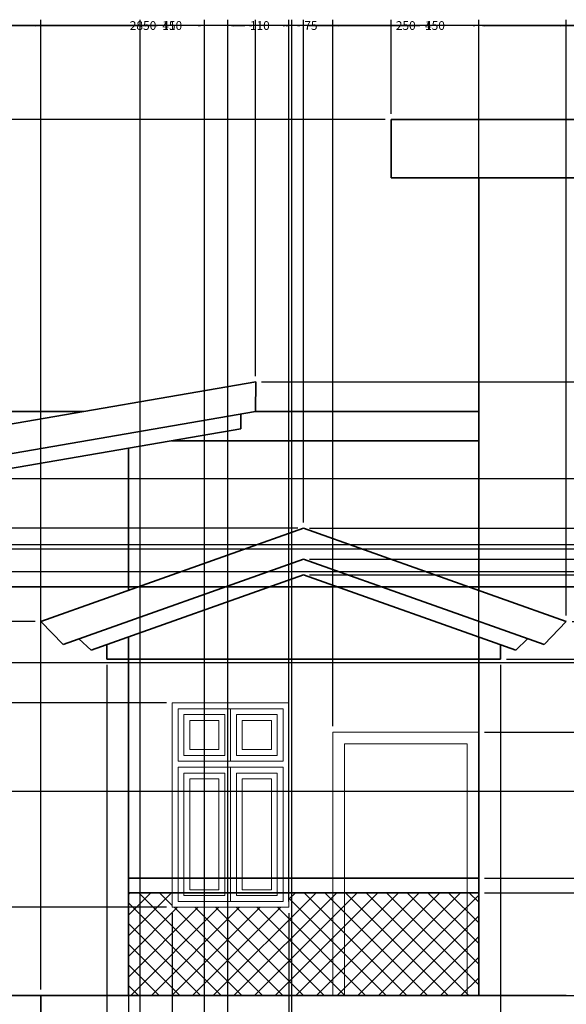
# Model space of a CAD drawing. Units: millimetres. Extents: x 937 to 4561, y 2711 to 5748.
# Tile 7 of 8: x 2543 to 3479, y 4062 to 5748. Entities that reach past the tile are written whole.
import ezdxf

# ---------------------------------------------------------------- set-up
doc = ezdxf.new("R2010")
doc.units = ezdxf.units.MM
doc.header["$MEASUREMENT"] = 0
for name, color, linetype, lineweight in [('A-ANNO-DIMS', 2, 'Continuous', 18), ('A-DOOR', 3, 'Continuous', 18), ('A-ELEV', 7, 'Continuous', 35), ('A-GLAZ', 4, 'Continuous', 18), ('A-ROOF', 1, 'Continuous', 35), ('A-WALL-PATT', 8, 'Continuous', 13)]:
    doc.layers.add(name, color=color, linetype=linetype, lineweight=lineweight)
doc.styles.get("Standard").update_dxf_attribs({"font": 'arial.ttf'})
doc.dimstyles.get("Standard").update_dxf_attribs({"dimtxt": 15, "dimasz": 10, "dimexe": 10, "dimexo": 10, "dimgap": 10, "dimtad": 0, "dimtih": 1, "dimtoh": 1, "dimdec": 0, "dimzin": 0, "dimdsep": 46, "dimtxsty": 'Standard', "dimcen": 5, "dimadec": 0, "dimazin": 0, "dimtfac": 1, "dimtdec": 0, "dimtofl": 0, "dimtmove": 0, "dimatfit": 3, "dimfxl": 1, "dimtolj": 1, "dimtzin": 0, "dimarcsym": 0})

# ---------------------------------------------------------------- blocks, each defined once
blk = doc.blocks.new('*D15')
at = {"layer": 'A-ANNO-DIMS', "color": 0, "lineweight": -2, "transparency": 16777216}
for p, q in [((1329.5, 4086.9), (1329.5, 5747.9)), ((1339.5, 5737.9), (2722, 5737.9)), ((4169.5, 5737.9), (2787, 5737.9)), ((4179.5, 5586.9), (4179.5, 5747.9))]:
    blk.add_line(p, q, dxfattribs=at)
at = {"layer": 'A-ANNO-DIMS', "color": 0, "transparency": 16777216}
for points in [[(1339.5, 5739.6), (1339.5, 5736.2), (1329.5, 5737.9)], [(4169.5, 5739.6), (4169.5, 5736.2), (4179.5, 5737.9)]]:
    blk.add_solid(points, dxfattribs=at)
at = {"layer": 'Defpoints', "color": 0, "transparency": 16777216}
for p in [(4179.5, 5737.9), (4179.5, 5576.9), (1329.5, 4076.9)]:
    blk.add_point(p, dxfattribs=at)
at = {"layer": 'A-ANNO-DIMS', "color": 0, "transparency": 16777216, "insert": (2754.5, 5737.9), "char_height": 15, "attachment_point": 5}
blk.add_mtext('\\A1;2850', dxfattribs=at)
blk = doc.blocks.new('*D16')
at = {"layer": 'A-ANNO-DIMS', "color": 0, "lineweight": -2, "transparency": 16777216}
for p, q in [((1329.5, 4859.2), (1329.5, 5747.9)), ((1339.5, 5737.9), (2106.8, 5737.9)), ((2937.4, 5737.9), (2170.2, 5737.9)), ((2947.4, 5137.7), (2947.4, 5747.9))]:
    blk.add_line(p, q, dxfattribs=at)
at = {"layer": 'A-ANNO-DIMS', "color": 0, "transparency": 16777216}
for points in [[(1339.5, 5739.6), (1339.5, 5736.2), (1329.5, 5737.9)], [(2937.4, 5739.6), (2937.4, 5736.2), (2947.4, 5737.9)]]:
    blk.add_solid(points, dxfattribs=at)
at = {"layer": 'Defpoints', "color": 0, "transparency": 16777216}
for p in [(2947.4, 5737.9), (2947.4, 5127.7), (1329.5, 4849.2)]:
    blk.add_point(p, dxfattribs=at)
at = {"layer": 'A-ANNO-DIMS', "color": 0, "transparency": 16777216, "insert": (2138.5, 5737.9), "char_height": 15, "attachment_point": 5}
blk.add_mtext('\\A1;1618', dxfattribs=at)
blk = doc.blocks.new('*D17')
at = {"layer": 'A-ANNO-DIMS', "color": 0, "lineweight": -2, "transparency": 16777216}
for p, q in [((3179.5, 5586.9), (3179.5, 5747.9)), ((3189.5, 5737.9), (3228.6, 5737.9)), ((3319.5, 5737.9), (3280.3, 5737.9)), ((3329.5, 5486.9), (3329.5, 5747.9))]:
    blk.add_line(p, q, dxfattribs=at)
at = {"layer": 'A-ANNO-DIMS', "color": 0, "transparency": 16777216}
for points in [[(3189.5, 5739.6), (3189.5, 5736.2), (3179.5, 5737.9)], [(3319.5, 5739.6), (3319.5, 5736.2), (3329.5, 5737.9)]]:
    blk.add_solid(points, dxfattribs=at)
at = {"layer": 'Defpoints', "color": 0, "transparency": 16777216}
for p in [(3329.5, 5737.9), (3179.5, 5576.9), (3329.5, 5476.9)]:
    blk.add_point(p, dxfattribs=at)
at = {"layer": 'A-ANNO-DIMS', "color": 0, "transparency": 16777216, "insert": (3254.5, 5737.9), "char_height": 15, "attachment_point": 5}
blk.add_mtext('\\A1;150', dxfattribs=at)
blk = doc.blocks.new('*D18')
at = {"layer": 'A-ANNO-DIMS', "color": 0, "lineweight": -2, "transparency": 16777216}
for p, q in [((3329.5, 5486.9), (3329.5, 5747.9)), ((3339.5, 5737.9), (3653, 5737.9)), ((4019.5, 5737.9), (3706, 5737.9)), ((4029.5, 5486.9), (4029.5, 5747.9))]:
    blk.add_line(p, q, dxfattribs=at)
at = {"layer": 'A-ANNO-DIMS', "color": 0, "transparency": 16777216}
for points in [[(3339.5, 5739.6), (3339.5, 5736.2), (3329.5, 5737.9)], [(4019.5, 5739.6), (4019.5, 5736.2), (4029.5, 5737.9)]]:
    blk.add_solid(points, dxfattribs=at)
at = {"layer": 'Defpoints', "color": 0, "transparency": 16777216}
for p in [(4029.5, 5737.9), (3329.5, 5476.9), (4029.5, 5476.9)]:
    blk.add_point(p, dxfattribs=at)
at = {"layer": 'A-ANNO-DIMS', "color": 0, "transparency": 16777216, "insert": (3679.5, 5737.9), "char_height": 15, "attachment_point": 5}
blk.add_mtext('\\A1;700', dxfattribs=at)
blk = doc.blocks.new('*D22')
at = {"layer": 'A-ANNO-DIMS', "color": 0, "lineweight": -2, "transparency": 16777216}
for p, q in [((2579.5, 4727.5), (2579.5, 5747.9)), ((2589.5, 5737.9), (2777.6, 5737.9)), ((3019.5, 5737.9), (2831.3, 5737.9)), ((3029.5, 4886.9), (3029.5, 5747.9))]:
    blk.add_line(p, q, dxfattribs=at)
at = {"layer": 'A-ANNO-DIMS', "color": 0, "transparency": 16777216}
for points in [[(2589.5, 5739.6), (2589.5, 5736.2), (2579.5, 5737.9)], [(3019.5, 5739.6), (3019.5, 5736.2), (3029.5, 5737.9)]]:
    blk.add_solid(points, dxfattribs=at)
at = {"layer": 'Defpoints', "color": 0, "transparency": 16777216}
for p in [(3029.5, 5737.9), (3029.5, 4876.9), (2579.5, 4717.5)]:
    blk.add_point(p, dxfattribs=at)
at = {"layer": 'A-ANNO-DIMS', "color": 0, "transparency": 16777216, "insert": (2804.5, 5737.9), "char_height": 15, "attachment_point": 5}
blk.add_mtext('\\A1;450', dxfattribs=at)
blk = doc.blocks.new('*D23')
at = {"layer": 'A-ANNO-DIMS', "color": 0, "lineweight": -2, "transparency": 16777216}
for p, q in [((3029.5, 4886.9), (3029.5, 5747.9)), ((3039.5, 5737.9), (3227.6, 5737.9)), ((3469.5, 5737.9), (3281.3, 5737.9)), ((3479.5, 4727.5), (3479.5, 5747.9))]:
    blk.add_line(p, q, dxfattribs=at)
at = {"layer": 'A-ANNO-DIMS', "color": 0, "transparency": 16777216}
for points in [[(3039.5, 5739.6), (3039.5, 5736.2), (3029.5, 5737.9)], [(3469.5, 5739.6), (3469.5, 5736.2), (3479.5, 5737.9)]]:
    blk.add_solid(points, dxfattribs=at)
at = {"layer": 'Defpoints', "color": 0, "transparency": 16777216}
for p in [(3479.5, 5737.9), (3029.5, 4876.9), (3479.5, 4717.5)]:
    blk.add_point(p, dxfattribs=at)
at = {"layer": 'A-ANNO-DIMS', "color": 0, "transparency": 16777216, "insert": (3254.5, 5737.9), "char_height": 15, "attachment_point": 5}
blk.add_mtext('\\A1;450', dxfattribs=at)
blk = doc.blocks.new('*D24')
at = {"layer": 'A-ANNO-DIMS', "color": 0, "lineweight": -2, "transparency": 16777216}
for p, q in [((2692.4, 4642.9), (2692.4, 2710.9)), ((3366.9, 4642.9), (3366.9, 2710.9)), ((2702.4, 2720.9), (2994.3, 2720.9)), ((3356.9, 2720.9), (3065.1, 2720.9))]:
    blk.add_line(p, q, dxfattribs=at)
at = {"layer": 'A-ANNO-DIMS', "color": 0, "transparency": 16777216}
for points in [[(2702.4, 2722.6), (2702.4, 2719.2), (2692.4, 2720.9)], [(3356.9, 2722.6), (3356.9, 2719.2), (3366.9, 2720.9)]]:
    blk.add_solid(points, dxfattribs=at)
at = {"layer": 'Defpoints', "color": 0, "transparency": 16777216}
for p in [(2692.4, 4652.9), (3366.9, 4652.9), (3366.9, 2720.9)]:
    blk.add_point(p, dxfattribs=at)
at = {"layer": 'A-ANNO-DIMS', "color": 0, "transparency": 16777216, "insert": (3029.7, 2720.9), "char_height": 15, "attachment_point": 5}
blk.add_mtext('\\A1;674.5', dxfattribs=at)
blk = doc.blocks.new('*D25')
at = {"layer": 'A-ANNO-DIMS', "color": 0, "lineweight": -2, "transparency": 16777216}
for p, q in [((3469.5, 5737.9), (3459.5, 5737.9)), ((3479.5, 5086.9), (3479.5, 5747.9)), ((3529.5, 5036.9), (3529.5, 5747.9)), ((3539.5, 5737.9), (3549.5, 5737.9))]:
    blk.add_line(p, q, dxfattribs=at)
at = {"layer": 'A-ANNO-DIMS', "color": 0, "transparency": 16777216}
for points in [[(3469.5, 5739.6), (3469.5, 5736.2), (3479.5, 5737.9)], [(3539.5, 5739.6), (3539.5, 5736.2), (3529.5, 5737.9)]]:
    blk.add_solid(points, dxfattribs=at)
at = {"layer": 'Defpoints', "color": 0, "transparency": 16777216}
for p in [(3529.5, 5737.9), (3479.5, 5076.9), (3529.5, 5026.9)]:
    blk.add_point(p, dxfattribs=at)
at = {"layer": 'A-ANNO-DIMS', "color": 0, "transparency": 16777216, "insert": (3504.5, 5737.9), "char_height": 15, "attachment_point": 5}
blk.add_mtext('\\A1;50', dxfattribs=at)
blk = doc.blocks.new('*D43')
at = {"layer": 'A-ANNO-DIMS', "color": 0, "lineweight": -2, "transparency": 16777216}
for p, q in [((1329.5, 4086.9), (1329.5, 5747.9)), ((1339.5, 5737.9), (1922.8, 5737.9)), ((2569.5, 5737.9), (1986.2, 5737.9)), ((2579.5, 4086.9), (2579.5, 5747.9))]:
    blk.add_line(p, q, dxfattribs=at)
at = {"layer": 'A-ANNO-DIMS', "color": 0, "transparency": 16777216}
for points in [[(1339.5, 5739.6), (1339.5, 5736.2), (1329.5, 5737.9)], [(2569.5, 5739.6), (2569.5, 5736.2), (2579.5, 5737.9)]]:
    blk.add_solid(points, dxfattribs=at)
at = {"layer": 'Defpoints', "color": 0, "transparency": 16777216}
for p in [(2579.5, 5737.9), (1329.5, 4076.9), (2579.5, 4076.9)]:
    blk.add_point(p, dxfattribs=at)
at = {"layer": 'A-ANNO-DIMS', "color": 0, "transparency": 16777216, "insert": (1954.5, 5737.9), "char_height": 15, "attachment_point": 5}
blk.add_mtext('\\A1;1250', dxfattribs=at)
blk = doc.blocks.new('*D49')
at = {"layer": 'A-ANNO-DIMS', "color": 0, "lineweight": -2, "transparency": 16777216}
for p, q in [((2729.5, 4242.9), (2729.5, 2710.9)), ((2804.5, 4217.9), (2804.5, 2710.9)), ((2719.5, 2720.9), (2709.5, 2720.9)), ((2814.5, 2720.9), (2824.5, 2720.9))]:
    blk.add_line(p, q, dxfattribs=at)
at = {"layer": 'A-ANNO-DIMS', "color": 0, "transparency": 16777216}
for points in [[(2719.5, 2722.6), (2719.5, 2719.2), (2729.5, 2720.9)], [(2814.5, 2722.6), (2814.5, 2719.2), (2804.5, 2720.9)]]:
    blk.add_solid(points, dxfattribs=at)
at = {"layer": 'Defpoints', "color": 0, "transparency": 16777216}
for p in [(2729.5, 4252.9), (2804.5, 4227.9), (2804.5, 2720.9)]:
    blk.add_point(p, dxfattribs=at)
at = {"layer": 'A-ANNO-DIMS', "color": 0, "transparency": 16777216, "insert": (2767, 2720.9), "char_height": 15, "attachment_point": 5}
blk.add_mtext('\\A1;75', dxfattribs=at)
blk = doc.blocks.new('*D50')
at = {"layer": 'A-ANNO-DIMS', "color": 0, "lineweight": -2, "transparency": 16777216}
for p, q in [((2804.5, 4217.9), (2804.5, 2710.9)), ((3004.5, 4217.9), (3004.5, 2710.9)), ((2814.5, 2720.9), (2877.8, 2720.9)), ((2994.5, 2720.9), (2931.2, 2720.9))]:
    blk.add_line(p, q, dxfattribs=at)
at = {"layer": 'A-ANNO-DIMS', "color": 0, "transparency": 16777216}
for points in [[(2814.5, 2722.6), (2814.5, 2719.2), (2804.5, 2720.9)], [(2994.5, 2722.6), (2994.5, 2719.2), (3004.5, 2720.9)]]:
    blk.add_solid(points, dxfattribs=at)
at = {"layer": 'Defpoints', "color": 0, "transparency": 16777216}
for p in [(2804.5, 4227.9), (3004.5, 4227.9), (3004.5, 2720.9)]:
    blk.add_point(p, dxfattribs=at)
at = {"layer": 'A-ANNO-DIMS', "color": 0, "transparency": 16777216, "insert": (2904.5, 2720.9), "char_height": 15, "attachment_point": 5}
blk.add_mtext('\\A1;200', dxfattribs=at)
blk = doc.blocks.new('*D51')
at = {"layer": 'A-ANNO-DIMS', "color": 0, "lineweight": -2, "transparency": 16777216}
for p, q in [((2994.5, 5737.9), (2984.5, 5737.9)), ((3004.5, 4237.9), (3004.5, 5747.9)), ((3079.5, 4537.9), (3079.5, 5747.9)), ((3089.5, 5737.9), (3099.5, 5737.9))]:
    blk.add_line(p, q, dxfattribs=at)
at = {"layer": 'A-ANNO-DIMS', "color": 0, "transparency": 16777216}
for points in [[(2994.5, 5739.6), (2994.5, 5736.2), (3004.5, 5737.9)], [(3089.5, 5739.6), (3089.5, 5736.2), (3079.5, 5737.9)]]:
    blk.add_solid(points, dxfattribs=at)
at = {"layer": 'Defpoints', "color": 0, "transparency": 16777216}
for p in [(3079.5, 5737.9), (3079.5, 4527.9), (3004.5, 4227.9)]:
    blk.add_point(p, dxfattribs=at)
at = {"layer": 'A-ANNO-DIMS', "color": 0, "transparency": 16777216, "insert": (3042, 5737.9), "char_height": 15, "attachment_point": 5}
blk.add_mtext('\\A1;75', dxfattribs=at)
blk = doc.blocks.new('*D52')
at = {"layer": 'A-ANNO-DIMS', "color": 0, "lineweight": -2, "transparency": 16777216}
for p, q in [((3079.5, 4537.9), (3079.5, 5747.9)), ((3089.5, 5737.9), (3177.8, 5737.9)), ((3319.5, 5737.9), (3231.2, 5737.9)), ((3329.5, 4537.9), (3329.5, 5747.9))]:
    blk.add_line(p, q, dxfattribs=at)
at = {"layer": 'A-ANNO-DIMS', "color": 0, "transparency": 16777216}
for points in [[(3089.5, 5739.6), (3089.5, 5736.2), (3079.5, 5737.9)], [(3319.5, 5739.6), (3319.5, 5736.2), (3329.5, 5737.9)]]:
    blk.add_solid(points, dxfattribs=at)
at = {"layer": 'Defpoints', "color": 0, "transparency": 16777216}
for p in [(3329.5, 5737.9), (3079.5, 4527.9), (3329.5, 4527.9)]:
    blk.add_point(p, dxfattribs=at)
at = {"layer": 'A-ANNO-DIMS', "color": 0, "transparency": 16777216, "insert": (3204.5, 5737.9), "char_height": 15, "attachment_point": 5}
blk.add_mtext('\\A1;250', dxfattribs=at)
blk = doc.blocks.new('*D53')
at = {"layer": 'A-ANNO-DIMS', "color": 0, "lineweight": -2, "transparency": 16777216}
for p, q in [((2749.5, 3666.9), (2749.5, 5747.9)), ((2759.5, 5737.9), (2778.6, 5737.9)), ((2849.5, 5737.9), (2830.3, 5737.9)), ((2859.5, 3666.9), (2859.5, 5747.9))]:
    blk.add_line(p, q, dxfattribs=at)
at = {"layer": 'A-ANNO-DIMS', "color": 0, "transparency": 16777216}
for points in [[(2759.5, 5739.6), (2759.5, 5736.2), (2749.5, 5737.9)], [(2849.5, 5739.6), (2849.5, 5736.2), (2859.5, 5737.9)]]:
    blk.add_solid(points, dxfattribs=at)
at = {"layer": 'Defpoints', "color": 0, "transparency": 16777216}
for p in [(2859.5, 5737.9), (2749.5, 3656.9), (2859.5, 3656.9)]:
    blk.add_point(p, dxfattribs=at)
at = {"layer": 'A-ANNO-DIMS', "color": 0, "transparency": 16777216, "insert": (2804.5, 5737.9), "char_height": 15, "attachment_point": 5}
blk.add_mtext('\\A1;110', dxfattribs=at)
blk = doc.blocks.new('*D54')
at = {"layer": 'A-ANNO-DIMS', "color": 0, "lineweight": -2, "transparency": 16777216}
for p, q in [((2899.5, 3666.9), (2899.5, 5747.9)), ((2909.5, 5737.9), (2928.6, 5737.9)), ((2999.5, 5737.9), (2980.3, 5737.9)), ((3009.5, 3666.9), (3009.5, 5747.9))]:
    blk.add_line(p, q, dxfattribs=at)
at = {"layer": 'A-ANNO-DIMS', "color": 0, "transparency": 16777216}
for points in [[(2909.5, 5739.6), (2909.5, 5736.2), (2899.5, 5737.9)], [(2999.5, 5739.6), (2999.5, 5736.2), (3009.5, 5737.9)]]:
    blk.add_solid(points, dxfattribs=at)
at = {"layer": 'Defpoints', "color": 0, "transparency": 16777216}
for p in [(3009.5, 5737.9), (2899.5, 3656.9), (3009.5, 3656.9)]:
    blk.add_point(p, dxfattribs=at)
at = {"layer": 'A-ANNO-DIMS', "color": 0, "transparency": 16777216, "insert": (2954.5, 5737.9), "char_height": 15, "attachment_point": 5}
blk.add_mtext('\\A1;110', dxfattribs=at)
blk = doc.blocks.new('*D63')
at = {"layer": 'A-ANNO-DIMS', "color": 0, "lineweight": -2, "transparency": 16777216}
for p, q in [((3169.5, 5576.9), (958.5, 5576.9)), ((968.5, 5566.9), (968.5, 5344.6)), ((968.5, 5086.9), (968.5, 5309.2)), ((1419.5, 5076.9), (958.5, 5076.9))]:
    blk.add_line(p, q, dxfattribs=at)
at = {"layer": 'A-ANNO-DIMS', "color": 0, "transparency": 16777216}
for points in [[(966.8, 5566.9), (970.2, 5566.9), (968.5, 5576.9)], [(966.8, 5086.9), (970.2, 5086.9), (968.5, 5076.9)]]:
    blk.add_solid(points, dxfattribs=at)
at = {"layer": 'Defpoints', "color": 0, "transparency": 16777216}
for p in [(968.5, 5576.9), (3179.5, 5576.9), (1429.5, 5076.9)]:
    blk.add_point(p, dxfattribs=at)
at = {"layer": 'A-ANNO-DIMS', "color": 0, "transparency": 16777216, "insert": (968.5, 5326.9), "char_height": 15, "attachment_point": 5}
blk.add_mtext('\\A1;500', dxfattribs=at)
blk = doc.blocks.new('*D68')
at = {"layer": 'A-ANNO-DIMS', "color": 0, "lineweight": -2, "transparency": 16777216}
for p, q in [((4490.5, 4812.8), (4490.5, 4822.8)), ((4490.5, 4822.8), (4500.5, 4822.8)), ((1364.5, 4802.8), (4500.5, 4802.8)), ((1364.5, 4777.4), (4500.5, 4777.4)), ((4490.5, 4767.4), (4490.5, 4757.4))]:
    blk.add_line(p, q, dxfattribs=at)
at = {"layer": 'A-ANNO-DIMS', "color": 0, "transparency": 16777216}
for points in [[(4488.8, 4812.8), (4492.2, 4812.8), (4490.5, 4802.8)], [(4488.8, 4767.4), (4492.2, 4767.4), (4490.5, 4777.4)]]:
    blk.add_solid(points, dxfattribs=at)
at = {"layer": 'Defpoints', "color": 0, "transparency": 16777216}
for p in [(1354.5, 4802.8), (4490.5, 4802.8), (1354.5, 4777.4)]:
    blk.add_point(p, dxfattribs=at)
at = {"layer": 'A-ANNO-DIMS', "color": 0, "transparency": 16777216, "insert": (4535.9, 4822.8), "char_height": 15, "attachment_point": 5}
blk.add_mtext('\\A1;25.37', dxfattribs=at)
blk = doc.blocks.new('*D69')
at = {"layer": 'A-ANNO-DIMS', "color": 0, "lineweight": -2, "transparency": 16777216}
for p, q in [((2957.4, 5127.7), (4500.5, 5127.7)), ((4490.5, 5117.7), (4490.5, 5006.1)), ((4490.5, 4859.2), (4490.5, 4970.8)), ((1339.5, 4849.2), (4500.5, 4849.2))]:
    blk.add_line(p, q, dxfattribs=at)
at = {"layer": 'A-ANNO-DIMS', "color": 0, "transparency": 16777216}
for points in [[(4488.8, 5117.7), (4492.2, 5117.7), (4490.5, 5127.7)], [(4488.8, 4859.2), (4492.2, 4859.2), (4490.5, 4849.2)]]:
    blk.add_solid(points, dxfattribs=at)
at = {"layer": 'Defpoints', "color": 0, "transparency": 16777216}
for p in [(2947.4, 5127.7), (4490.5, 5127.7), (1329.5, 4849.2)]:
    blk.add_point(p, dxfattribs=at)
at = {"layer": 'A-ANNO-DIMS', "color": 0, "transparency": 16777216, "insert": (4490.5, 4988.5), "char_height": 15, "attachment_point": 5}
blk.add_mtext('\\A1;278.45', dxfattribs=at)
blk = doc.blocks.new('*D75')
at = {"layer": 'A-ANNO-DIMS', "color": 0, "lineweight": -2, "transparency": 16777216}
for p, q in [((1829.5, 4646.9), (4500.5, 4646.9)), ((4490.5, 4636.9), (4490.5, 4554.6)), ((4490.5, 4436.9), (4490.5, 4519.2)), ((1829.5, 4426.9), (4500.5, 4426.9))]:
    blk.add_line(p, q, dxfattribs=at)
at = {"layer": 'A-ANNO-DIMS', "color": 0, "transparency": 16777216}
for points in [[(4488.8, 4636.9), (4492.2, 4636.9), (4490.5, 4646.9)], [(4488.8, 4436.9), (4492.2, 4436.9), (4490.5, 4426.9)]]:
    blk.add_solid(points, dxfattribs=at)
at = {"layer": 'Defpoints', "color": 0, "transparency": 16777216}
for p in [(1819.5, 4646.9), (4490.5, 4646.9), (1819.5, 4426.9)]:
    blk.add_point(p, dxfattribs=at)
at = {"layer": 'A-ANNO-DIMS', "color": 0, "transparency": 16777216, "insert": (4490.5, 4536.9), "char_height": 15, "attachment_point": 5}
blk.add_mtext('\\A1;220', dxfattribs=at)
blk = doc.blocks.new('*D76')
at = {"layer": 'A-ANNO-DIMS', "color": 0, "lineweight": -2, "transparency": 16777216}
for p, q in [((1829.5, 4776.9), (4500.5, 4776.9)), ((4490.5, 4766.9), (4490.5, 4729.6)), ((4490.5, 4656.9), (4490.5, 4694.2)), ((1829.5, 4646.9), (4500.5, 4646.9))]:
    blk.add_line(p, q, dxfattribs=at)
at = {"layer": 'A-ANNO-DIMS', "color": 0, "transparency": 16777216}
for points in [[(4488.8, 4766.9), (4492.2, 4766.9), (4490.5, 4776.9)], [(4488.8, 4656.9), (4492.2, 4656.9), (4490.5, 4646.9)]]:
    blk.add_solid(points, dxfattribs=at)
at = {"layer": 'Defpoints', "color": 0, "transparency": 16777216}
for p in [(1819.5, 4776.9), (4490.5, 4776.9), (1819.5, 4646.9)]:
    blk.add_point(p, dxfattribs=at)
at = {"layer": 'A-ANNO-DIMS', "color": 0, "transparency": 16777216, "insert": (4490.5, 4711.9), "char_height": 15, "attachment_point": 5}
blk.add_mtext('\\A1;130', dxfattribs=at)
blk = doc.blocks.new('*D78')
at = {"layer": 'A-ANNO-DIMS', "color": 0, "lineweight": -2, "transparency": 16777216}
for p, q in [((2439.5, 4962.4), (4500.5, 4962.4)), ((4490.5, 4952.4), (4490.5, 4919.9)), ((4490.5, 4852), (4490.5, 4884.5)), ((1739.5, 4842), (4500.5, 4842))]:
    blk.add_line(p, q, dxfattribs=at)
at = {"layer": 'A-ANNO-DIMS', "color": 0, "transparency": 16777216}
for points in [[(4488.8, 4952.4), (4492.2, 4952.4), (4490.5, 4962.4)], [(4488.8, 4852), (4492.2, 4852), (4490.5, 4842)]]:
    blk.add_solid(points, dxfattribs=at)
at = {"layer": 'Defpoints', "color": 0, "transparency": 16777216}
for p in [(2429.5, 4962.4), (4490.5, 4962.4), (1729.5, 4842)]:
    blk.add_point(p, dxfattribs=at)
at = {"layer": 'A-ANNO-DIMS', "color": 0, "transparency": 16777216, "insert": (4490.5, 4902.2), "char_height": 15, "attachment_point": 5}
blk.add_mtext('\\A1;120.47', dxfattribs=at)
blk = doc.blocks.new('*D79')
at = {"layer": 'A-ANNO-DIMS', "color": 0, "lineweight": -2, "transparency": 16777216}
for p, q in [((3019.5, 4876.9), (958.5, 4876.9)), ((968.5, 4866.9), (968.5, 4814.8)), ((968.5, 4727.5), (968.5, 4779.5)), ((2569.5, 4717.5), (958.5, 4717.5))]:
    blk.add_line(p, q, dxfattribs=at)
at = {"layer": 'A-ANNO-DIMS', "color": 0, "transparency": 16777216}
for points in [[(966.8, 4866.9), (970.2, 4866.9), (968.5, 4876.9)], [(966.8, 4727.5), (970.2, 4727.5), (968.5, 4717.5)]]:
    blk.add_solid(points, dxfattribs=at)
at = {"layer": 'Defpoints', "color": 0, "transparency": 16777216}
for p in [(968.5, 4876.9), (3029.5, 4876.9), (2579.5, 4717.5)]:
    blk.add_point(p, dxfattribs=at)
at = {"layer": 'A-ANNO-DIMS', "color": 0, "transparency": 16777216, "insert": (968.5, 4797.2), "char_height": 15, "attachment_point": 5}
blk.add_mtext('\\A1;159.44', dxfattribs=at)
blk = doc.blocks.new('*D80')
at = {"layer": 'A-ANNO-DIMS', "color": 0, "lineweight": -2, "transparency": 16777216}
for p, q in [((3039.5, 4876.9), (4500.5, 4876.9)), ((4490.5, 4866.9), (4490.5, 4833.9)), ((3039.5, 4823.9), (4500.5, 4823.9)), ((4490.5, 4823.9), (4490.5, 4813.9)), ((4490.5, 4813.9), (4480.5, 4813.9))]:
    blk.add_line(p, q, dxfattribs=at)
at = {"layer": 'A-ANNO-DIMS', "color": 0, "transparency": 16777216}
for points in [[(4488.8, 4866.9), (4492.2, 4866.9), (4490.5, 4876.9)], [(4488.8, 4833.9), (4492.2, 4833.9), (4490.5, 4823.9)]]:
    blk.add_solid(points, dxfattribs=at)
at = {"layer": 'Defpoints', "color": 0, "transparency": 16777216}
for p in [(3029.5, 4876.9), (3029.5, 4823.9), (4490.5, 4823.9)]:
    blk.add_point(p, dxfattribs=at)
at = {"layer": 'A-ANNO-DIMS', "color": 0, "transparency": 16777216, "insert": (4445.1, 4813.9), "char_height": 15, "attachment_point": 5}
blk.add_mtext('\\A1;53.05', dxfattribs=at)
blk = doc.blocks.new('*D81')
at = {"layer": 'A-ANNO-DIMS', "color": 0, "lineweight": -2, "transparency": 16777216}
for p, q in [((4490.5, 4833.9), (4490.5, 4843.9)), ((3039.5, 4823.9), (4500.5, 4823.9)), ((3039.5, 4797.3), (4500.5, 4797.3)), ((4490.5, 4777.3), (4480.5, 4777.3)), ((4490.5, 4787.3), (4490.5, 4777.3))]:
    blk.add_line(p, q, dxfattribs=at)
at = {"layer": 'A-ANNO-DIMS', "color": 0, "transparency": 16777216}
for points in [[(4488.8, 4833.9), (4492.2, 4833.9), (4490.5, 4823.9)], [(4488.8, 4787.3), (4492.2, 4787.3), (4490.5, 4797.3)]]:
    blk.add_solid(points, dxfattribs=at)
at = {"layer": 'Defpoints', "color": 0, "transparency": 16777216}
for p in [(3029.5, 4823.9), (3029.5, 4797.3), (4490.5, 4797.3)]:
    blk.add_point(p, dxfattribs=at)
at = {"layer": 'A-ANNO-DIMS', "color": 0, "transparency": 16777216, "insert": (4439.2, 4777.3), "char_height": 15, "attachment_point": 5}
blk.add_mtext('\\A1;26.523', dxfattribs=at)
blk = doc.blocks.new('*D86')
at = {"layer": 'A-ANNO-DIMS', "color": 0, "lineweight": -2, "transparency": 16777216}
for p, q in [((968.5, 4076.9), (968.5, 4086.9)), ((968.5, 4086.9), (978.5, 4086.9)), ((2569.5, 4076.9), (958.5, 4076.9)), ((968.5, 4036.9), (968.5, 4066.9)), ((2569.5, 4026.9), (958.5, 4026.9))]:
    blk.add_line(p, q, dxfattribs=at)
at = {"layer": 'A-ANNO-DIMS', "color": 0, "transparency": 16777216}
for points in [[(966.8, 4066.9), (970.2, 4066.9), (968.5, 4076.9)], [(966.8, 4036.9), (970.2, 4036.9), (968.5, 4026.9)]]:
    blk.add_solid(points, dxfattribs=at)
at = {"layer": 'Defpoints', "color": 0, "transparency": 16777216}
for p in [(968.5, 4076.9), (2579.5, 4076.9), (2579.5, 4026.9)]:
    blk.add_point(p, dxfattribs=at)
at = {"layer": 'A-ANNO-DIMS', "color": 0, "transparency": 16777216, "insert": (999.2, 4086.9), "char_height": 15, "attachment_point": 5}
blk.add_mtext('\\A1;50', dxfattribs=at)
blk = doc.blocks.new('*D87')
at = {"layer": 'A-ANNO-DIMS', "color": 0, "lineweight": -2, "transparency": 16777216}
for p, q in [((2794.5, 4227.9), (958.5, 4227.9)), ((968.5, 4217.9), (968.5, 4170.1)), ((968.5, 4086.9), (968.5, 4134.7)), ((2719.5, 4076.9), (958.5, 4076.9))]:
    blk.add_line(p, q, dxfattribs=at)
at = {"layer": 'A-ANNO-DIMS', "color": 0, "transparency": 16777216}
for points in [[(966.8, 4217.9), (970.2, 4217.9), (968.5, 4227.9)], [(966.8, 4086.9), (970.2, 4086.9), (968.5, 4076.9)]]:
    blk.add_solid(points, dxfattribs=at)
at = {"layer": 'Defpoints', "color": 0, "transparency": 16777216}
for p in [(968.5, 4227.9), (2804.5, 4227.9), (2729.5, 4076.9)]:
    blk.add_point(p, dxfattribs=at)
at = {"layer": 'A-ANNO-DIMS', "color": 0, "transparency": 16777216, "insert": (968.5, 4152.4), "char_height": 15, "attachment_point": 5}
blk.add_mtext('\\A1;151', dxfattribs=at)
blk = doc.blocks.new('*D88')
at = {"layer": 'A-ANNO-DIMS', "color": 0, "lineweight": -2, "transparency": 16777216}
for p, q in [((3339.5, 4252.9), (4500.5, 4252.9)), ((4490.5, 4242.9), (4490.5, 4182.6)), ((4490.5, 4086.9), (4490.5, 4147.2)), ((3339.5, 4076.9), (4500.5, 4076.9))]:
    blk.add_line(p, q, dxfattribs=at)
at = {"layer": 'A-ANNO-DIMS', "color": 0, "transparency": 16777216}
for points in [[(4488.8, 4242.9), (4492.2, 4242.9), (4490.5, 4252.9)], [(4488.8, 4086.9), (4492.2, 4086.9), (4490.5, 4076.9)]]:
    blk.add_solid(points, dxfattribs=at)
at = {"layer": 'Defpoints', "color": 0, "transparency": 16777216}
for p in [(3329.5, 4252.9), (4490.5, 4252.9), (3329.5, 4076.9)]:
    blk.add_point(p, dxfattribs=at)
at = {"layer": 'A-ANNO-DIMS', "color": 0, "transparency": 16777216, "insert": (4490.5, 4164.9), "char_height": 15, "attachment_point": 5}
blk.add_mtext('\\A1;176', dxfattribs=at)
blk = doc.blocks.new('*D89')
at = {"layer": 'A-ANNO-DIMS', "color": 0, "lineweight": -2, "transparency": 16777216}
for p, q in [((4490.5, 4287.9), (4490.5, 4297.9)), ((4490.5, 4297.9), (4500.5, 4297.9)), ((3339.5, 4277.9), (4500.5, 4277.9)), ((3339.5, 4252.9), (4500.5, 4252.9)), ((4490.5, 4242.9), (4490.5, 4232.9))]:
    blk.add_line(p, q, dxfattribs=at)
at = {"layer": 'A-ANNO-DIMS', "color": 0, "transparency": 16777216}
for points in [[(4488.8, 4287.9), (4492.2, 4287.9), (4490.5, 4277.9)], [(4488.8, 4242.9), (4492.2, 4242.9), (4490.5, 4252.9)]]:
    blk.add_solid(points, dxfattribs=at)
at = {"layer": 'Defpoints', "color": 0, "transparency": 16777216}
for p in [(3329.5, 4277.9), (4490.5, 4277.9), (3329.5, 4252.9)]:
    blk.add_point(p, dxfattribs=at)
at = {"layer": 'A-ANNO-DIMS', "color": 0, "transparency": 16777216, "insert": (4521.4, 4297.9), "char_height": 15, "attachment_point": 5}
blk.add_mtext('\\A1;25', dxfattribs=at)
blk = doc.blocks.new('*D90')
at = {"layer": 'A-ANNO-DIMS', "color": 0, "lineweight": -2, "transparency": 16777216}
for p, q in [((3339.5, 4527.9), (4500.5, 4527.9)), ((4490.5, 4517.9), (4490.5, 4420.6)), ((4490.5, 4287.9), (4490.5, 4385.2)), ((3339.5, 4277.9), (4500.5, 4277.9))]:
    blk.add_line(p, q, dxfattribs=at)
at = {"layer": 'A-ANNO-DIMS', "color": 0, "transparency": 16777216}
for points in [[(4488.8, 4517.9), (4492.2, 4517.9), (4490.5, 4527.9)], [(4488.8, 4287.9), (4492.2, 4287.9), (4490.5, 4277.9)]]:
    blk.add_solid(points, dxfattribs=at)
at = {"layer": 'Defpoints', "color": 0, "transparency": 16777216}
for p in [(3329.5, 4527.9), (4490.5, 4527.9), (3329.5, 4277.9)]:
    blk.add_point(p, dxfattribs=at)
at = {"layer": 'A-ANNO-DIMS', "color": 0, "transparency": 16777216, "insert": (4490.5, 4402.9), "char_height": 15, "attachment_point": 5}
blk.add_mtext('\\A1;250', dxfattribs=at)
blk = doc.blocks.new('*D91')
at = {"layer": 'A-ANNO-DIMS', "color": 0, "lineweight": -2, "transparency": 16777216}
for p, q in [((3376.9, 4652.9), (4500.5, 4652.9)), ((4490.5, 4642.9), (4490.5, 4608.1)), ((4490.5, 4537.9), (4490.5, 4572.7)), ((3339.5, 4527.9), (4500.5, 4527.9))]:
    blk.add_line(p, q, dxfattribs=at)
at = {"layer": 'A-ANNO-DIMS', "color": 0, "transparency": 16777216}
for points in [[(4488.8, 4642.9), (4492.2, 4642.9), (4490.5, 4652.9)], [(4488.8, 4537.9), (4492.2, 4537.9), (4490.5, 4527.9)]]:
    blk.add_solid(points, dxfattribs=at)
at = {"layer": 'Defpoints', "color": 0, "transparency": 16777216}
for p in [(3366.9, 4652.9), (4490.5, 4652.9), (3329.5, 4527.9)]:
    blk.add_point(p, dxfattribs=at)
at = {"layer": 'A-ANNO-DIMS', "color": 0, "transparency": 16777216, "insert": (4490.5, 4590.4), "char_height": 15, "attachment_point": 5}
blk.add_mtext('\\A1;125', dxfattribs=at)
blk = doc.blocks.new('*D92')
at = {"layer": 'A-ANNO-DIMS', "color": 0, "lineweight": -2, "transparency": 16777216}
for p, q in [((4490.5, 4717.5), (4490.5, 4727.5)), ((4490.5, 4727.5), (4500.5, 4727.5)), ((3489.5, 4717.5), (4500.5, 4717.5)), ((4490.5, 4662.9), (4490.5, 4707.5)), ((3376.9, 4652.9), (4500.5, 4652.9))]:
    blk.add_line(p, q, dxfattribs=at)
at = {"layer": 'A-ANNO-DIMS', "color": 0, "transparency": 16777216}
for points in [[(4488.8, 4707.5), (4492.2, 4707.5), (4490.5, 4717.5)], [(4488.8, 4662.9), (4492.2, 4662.9), (4490.5, 4652.9)]]:
    blk.add_solid(points, dxfattribs=at)
at = {"layer": 'Defpoints', "color": 0, "transparency": 16777216}
for p in [(3479.5, 4717.5), (4490.5, 4717.5), (3366.9, 4652.9)]:
    blk.add_point(p, dxfattribs=at)
at = {"layer": 'A-ANNO-DIMS', "color": 0, "transparency": 16777216, "insert": (4535.8, 4727.5), "char_height": 15, "attachment_point": 5}
blk.add_mtext('\\A1;64.56', dxfattribs=at)
blk = doc.blocks.new('*D93')
at = {"layer": 'A-ANNO-DIMS', "color": 0, "lineweight": -2, "transparency": 16777216}
for p, q in [((2794.5, 4577.9), (958.5, 4577.9)), ((968.5, 4567.9), (968.5, 4420.6)), ((968.5, 4237.9), (968.5, 4385.2)), ((2794.5, 4227.9), (958.5, 4227.9))]:
    blk.add_line(p, q, dxfattribs=at)
at = {"layer": 'A-ANNO-DIMS', "color": 0, "transparency": 16777216}
for points in [[(966.8, 4567.9), (970.2, 4567.9), (968.5, 4577.9)], [(966.8, 4237.9), (970.2, 4237.9), (968.5, 4227.9)]]:
    blk.add_solid(points, dxfattribs=at)
at = {"layer": 'Defpoints', "color": 0, "transparency": 16777216}
for p in [(968.5, 4577.9), (2804.5, 4577.9), (2804.5, 4227.9)]:
    blk.add_point(p, dxfattribs=at)
at = {"layer": 'A-ANNO-DIMS', "color": 0, "transparency": 16777216, "insert": (968.5, 4402.9), "char_height": 15, "attachment_point": 5}
blk.add_mtext('\\A1;350', dxfattribs=at)

msp = doc.modelspace()

# ---------------------------------------------------------------- hatches: boundary and pattern name
at = {"layer": 'A-WALL-PATT'}
h = msp.add_hatch(dxfattribs=at)
h.set_pattern_fill('ANSI37', color=256, scale=200)
h.paths.add_polyline_path([(3309.4852, 4252.9001), (3099.4852, 4252.9001), (3099.4852, 4076.9013), (3309.4852, 4076.9013)])
h.paths.add_polyline_path([(3329.4852, 4252.9001), (3309.4852, 4252.9001), (3309.4852, 4076.9013), (3329.4852, 4076.9013)])
h.paths.add_polyline_path([(3099.4852, 4252.9001), (3079.4852, 4252.9001), (3079.4852, 4076.9013), (3099.4852, 4076.9013)])
h.paths.add_polyline_path([(3079.4852, 4252.9001), (3004.4852, 4252.9001), (3004.4852, 4227.9047), (2804.4852, 4227.9047), (2804.4852, 4252.9001), (2729.4852, 4252.9001), (2729.4852, 4076.9013), (3079.4852, 4076.9013)])

# ---------------------------------------------------------------- linework, layer by layer
at = {"layer": 'A-DOOR'}
for p, q in [((3079.4852, 4076.9013), (3079.4852, 4527.9001)), ((3079.4852, 4527.9001), (3329.4852, 4527.9001)), ((3099.4852, 4076.9013), (3099.4852, 4507.9001)), ((3099.4852, 4507.9001), (3309.4852, 4507.9001)), ((3309.4852, 4076.9013), (3309.4852, 4507.9001))]:
    msp.add_line(p, q, dxfattribs=at)
at = {"layer": 'A-ELEV'}
for p, q in [((3929.4852, 5576.9013), (3179.4852, 5576.9013)), ((3179.4852, 5576.9013), (3179.4852, 5476.9013)), ((3179.4852, 5476.9013), (4179.4852, 5476.9013)), ((3329.4852, 4770.6073), (3329.4852, 5476.9013)), ((2947.4456, 5127.6834), (2947.1723, 5076.9013)), ((2947.1723, 5076.9013), (3329.4852, 5076.9013)), ((2804.041, 5026.9013), (3329.4852, 5026.9013)), ((2729.4852, 4770.6073), (2729.4852, 5014.0705)), ((2729.4852, 4076.9013), (2729.4852, 4691.0388)), ((3329.4852, 4076.9013), (3329.4852, 4691.0388)), ((2729.4852, 4277.9001), (3329.4852, 4277.9001)), ((2729.4852, 4252.9001), (3329.4852, 4252.9001)), ((1429.4852, 4076.9013), (3479.4852, 4076.9013)), ((2729.4852, 4076.9013), (2479.4852, 4076.9013)), ((2729.4852, 4076.9013), (2579.4852, 4076.9013)), ((2579.4852, 4076.9013), (2579.4852, 3976.9013)), ((3329.4852, 4076.9013), (3479.4852, 4076.9013))]:
    msp.add_line(p, q, dxfattribs=at)
at = {"layer": 'A-GLAZ'}
for p, q in [((2804.4852, 4252.9001), (2804.4852, 4577.9047)), ((2804.4852, 4577.9047), (3004.4852, 4577.9047)), ((2804.4852, 4577.9047), (3004.4852, 4577.9047)), ((2804.4852, 4227.9047), (2804.4852, 4577.9047)), ((3004.4852, 4252.9001), (3004.4852, 4577.9047)), ((3004.4852, 4577.9047), (3004.4852, 4227.9047)), ((3004.4852, 4227.9047), (2804.4852, 4227.9047))]:
    msp.add_line(p, q, dxfattribs=at)
for points in [[(2814.4852, 4567.9047), (2904.4852, 4567.9047), (2904.4852, 4477.9047), (2814.4852, 4477.9047)], [(2824.4852, 4557.9047), (2894.4852, 4557.9047), (2894.4852, 4487.9047), (2824.4852, 4487.9047)], [(2904.4852, 4567.9047), (2994.4852, 4567.9047), (2994.4852, 4477.9047), (2904.4852, 4477.9047)], [(2914.4852, 4557.9047), (2984.4852, 4557.9047), (2984.4852, 4487.9047), (2914.4852, 4487.9047)], [(2834.4852, 4547.9047), (2884.4852, 4547.9047), (2884.4852, 4497.9047), (2834.4852, 4497.9047)], [(2924.4852, 4547.9047), (2974.4852, 4547.9047), (2974.4852, 4497.9047), (2924.4852, 4497.9047)], [(2814.4852, 4467.9047), (2904.4852, 4467.9047), (2904.4852, 4237.9047), (2814.4852, 4237.9047)], [(2824.4852, 4457.9047), (2894.4852, 4457.9047), (2894.4852, 4247.9047), (2824.4852, 4247.9047)], [(2904.4852, 4467.9047), (2994.4852, 4467.9047), (2994.4852, 4237.9047), (2904.4852, 4237.9047)], [(2914.4852, 4457.9047), (2984.4852, 4457.9047), (2984.4852, 4247.9047), (2914.4852, 4247.9047)], [(2834.4852, 4447.9047), (2884.4852, 4447.9047), (2884.4852, 4257.9047), (2834.4852, 4257.9047)], [(2924.4852, 4447.9047), (2974.4852, 4447.9047), (2974.4852, 4257.9047), (2924.4852, 4257.9047)]]:
    msp.add_lwpolyline(points, close=True, dxfattribs=at)
at = {"layer": 'A-ROOF'}
for p, q in [((2947.4456, 5127.6834), (1329.4852, 4849.2371)), ((2947.1723, 5076.9013), (1329.4852, 4798.5021)), ((1429.4852, 5076.9013), (2652.3676, 5076.9013)), ((2922.1488, 5072.5949), (2922.0122, 5047.2038)), ((2922.0122, 5047.2038), (1354.4852, 4777.437)), ((3029.4852, 4876.9013), (2579.4852, 4717.4604)), ((3029.4852, 4876.9013), (3479.4852, 4717.4604)), ((3029.4852, 4823.8556), (2617.587, 4677.9146)), ((3029.4852, 4823.8556), (3441.837, 4677.7539)), ((3029.4852, 4797.3328), (2665.5674, 4668.3919)), ((3029.4852, 4797.3328), (3393.1734, 4668.4733)), ((2579.4852, 4717.4604), (2617.587, 4677.9146)), ((3479.4852, 4717.4604), (3441.837, 4677.7539)), ((2665.5674, 4668.3919), (2644.3786, 4687.4073)), ((3393.1734, 4668.4733), (3413.0537, 4687.9522)), ((2692.4029, 4677.9001), (2692.4029, 4652.9001)), ((3366.9387, 4677.7685), (3366.9387, 4652.9001)), ((2692.4029, 4652.9001), (3366.9387, 4652.9001))]:
    msp.add_line(p, q, dxfattribs=at)

# ---------------------------------------------------------------- dimensions: what is measured, and where the dimension line sits
at = {"layer": 'A-ANNO-DIMS'}
for base, p1, p2, override, picture, middle in [((4179.4852, 5737.9013), (1329.4852, 4076.9013), (4179.4852, 5576.9013), {"dimdec": 0, "dimlfac": 1, "dimrnd": 0, "dimzin": 0, "dimdsep": 46, "dimlunit": 2}, '*D15', (2754.4852, 5737.9013)), ((2947.4456, 5737.9013), (1329.4852, 4849.2371), (2947.4456, 5127.6834), {"dimdec": 0, "dimlfac": 1, "dimrnd": 0, "dimzin": 0, "dimdsep": 46, "dimlunit": 2}, '*D16', (2138.4654, 5737.9013)), ((2579.4852, 5737.9013), (1329.4852, 4076.9013), (2579.4852, 4076.9013), {"dimdec": 0, "dimlfac": 1, "dimrnd": 0, "dimzin": 0, "dimdsep": 46, "dimlunit": 2}, '*D43', (1954.4852, 5737.9013)), ((3029.4852, 5737.9013), (2579.4852, 4717.4604), (3029.4852, 4876.9013), {"dimdec": 0, "dimlfac": 1, "dimrnd": 0, "dimzin": 0, "dimdsep": 46, "dimlunit": 2}, '*D22', (2804.4852, 5737.9013)), ((2859.4852, 5737.9013), (2749.4852, 3656.9013), (2859.4852, 3656.9013), {"dimdec": 0, "dimlfac": 1, "dimrnd": 0, "dimzin": 0, "dimdsep": 46, "dimlunit": 2}, '*D53', (2804.4852, 5737.9013)), ((3009.4852, 5737.9013), (2899.4852, 3656.9013), (3009.4852, 3656.9013), {"dimdec": 0, "dimlfac": 1, "dimrnd": 0, "dimzin": 0, "dimdsep": 46, "dimlunit": 2}, '*D54', (2954.4852, 5737.9013)), ((3079.4852, 5737.9013), (3004.4852, 4227.9047), (3079.4852, 4527.9001), {"dimdec": 0, "dimlfac": 1, "dimrnd": 0, "dimzin": 0, "dimdsep": 46, "dimlunit": 2}, '*D51', (3041.9852, 5737.9013)), ((3479.4852, 5737.9013), (3029.4852, 4876.9013), (3479.4852, 4717.4604), {"dimdec": 0, "dimlfac": 1, "dimrnd": 0, "dimzin": 0, "dimdsep": 46, "dimlunit": 2}, '*D23', (3254.4852, 5737.9013)), ((3329.4852, 5737.9013), (3079.4852, 4527.9001), (3329.4852, 4527.9001), {"dimdec": 0, "dimlfac": 1, "dimrnd": 0, "dimzin": 0, "dimdsep": 46, "dimlunit": 2}, '*D52', (3204.4852, 5737.9013)), ((3329.4852, 5737.9013), (3179.4852, 5576.9013), (3329.4852, 5476.9013), {"dimdec": 0, "dimlfac": 1, "dimrnd": 0, "dimzin": 0, "dimdsep": 46, "dimlunit": 2}, '*D17', (3254.4852, 5737.9013)), ((4029.4852, 5737.9013), (3329.4852, 5476.9013), (4029.4852, 5476.9013), {"dimdec": 0, "dimlfac": 1, "dimrnd": 0, "dimzin": 0, "dimdsep": 46, "dimlunit": 2}, '*D18', (3679.4852, 5737.9013)), ((3529.4852, 5737.9013), (3479.4852, 5076.9013), (3529.4852, 5026.9013), {"dimdec": 0, "dimlfac": 1, "dimrnd": 0, "dimzin": 0, "dimdsep": 46, "dimlunit": 2}, '*D25', (3504.4852, 5737.9013)), ((3366.9387, 2720.9013), (2692.4029, 4652.9001), (3366.9387, 4652.9001), {"dimdec": 1, "dimlfac": 1, "dimrnd": 0, "dimzin": 0, "dimdsep": 46, "dimlunit": 2}, '*D24', (3029.6708, 2720.9013)), ((2804.4852, 2720.9013), (2729.4852, 4252.9001), (2804.4852, 4227.9047), {"dimdec": 0, "dimlfac": 1, "dimrnd": 0, "dimzin": 0, "dimdsep": 46, "dimlunit": 2}, '*D49', (2766.9852, 2720.9013)), ((3004.4852, 2720.9013), (2804.4852, 4227.9047), (3004.4852, 4227.9047), {"dimdec": 0, "dimlfac": 1, "dimrnd": 0, "dimzin": 0, "dimdsep": 46, "dimlunit": 2}, '*D50', (2904.4852, 2720.9013))]:
    dim = msp.add_linear_dim(base=base, p1=p1, p2=p2, dimstyle='Standard', override=override, dxfattribs=at)
    dim.commit()
    dim.dimension.update_dxf_attribs({"geometry": picture, "text_midpoint": middle})
for base, p1, p2, override, picture, middle in [((968.4852, 5576.9013), (1429.4852, 5076.9013), (3179.4852, 5576.9013), {"dimdec": 0, "dimlfac": 1, "dimrnd": 0, "dimzin": 0, "dimdsep": 46, "dimlunit": 2}, '*D63', (968.4852, 5326.9013)), ((4490.4852, 5127.6834), (1329.4852, 4849.2371), (2947.4456, 5127.6834), {"dimdec": 2, "dimlfac": 1, "dimrnd": 0, "dimzin": 0, "dimdsep": 46, "dimlunit": 2}, '*D69', (4490.4852, 4988.4602)), ((4490.4852, 4962.4414), (1729.4852, 4841.9734), (2429.4852, 4962.4414), {"dimdec": 2, "dimlfac": 1, "dimrnd": 0, "dimzin": 0, "dimdsep": 46, "dimlunit": 2}, '*D78', (4490.4852, 4902.2074)), ((968.4852, 4876.9013), (2579.4852, 4717.4604), (3029.4852, 4876.9013), {"dimdec": 2, "dimlfac": 1, "dimrnd": 0, "dimzin": 0, "dimdsep": 46, "dimlunit": 2}, '*D79', (968.4852, 4797.1808)), ((4490.4852, 4823.8556), (3029.4852, 4876.9013), (3029.4852, 4823.8556), {"dimdec": 2, "dimlfac": 1, "dimrnd": 0, "dimzin": 0, "dimdsep": 46, "dimlunit": 2}, '*D80', (4445.1203, 4813.8556)), ((4490.4852, 4797.3328), (3029.4852, 4823.8556), (3029.4852, 4797.3328), {"dimdec": 3, "dimlfac": 1, "dimrnd": 0, "dimzin": 0, "dimdsep": 46, "dimlunit": 2}, '*D81', (4439.2216, 4777.3328)), ((4490.4852, 4802.8045), (1354.4852, 4777.437), (1354.4852, 4802.8045), {"dimdec": 2, "dimlfac": 1, "dimrnd": 0, "dimzin": 0, "dimdsep": 46, "dimlunit": 2}, '*D68', (4535.9218, 4822.8045)), ((4490.4852, 4776.9013), (1819.4852, 4646.9013), (1819.4852, 4776.9013), {"dimdec": 0, "dimlfac": 1, "dimrnd": 0, "dimzin": 0, "dimdsep": 46, "dimlunit": 2}, '*D76', (4490.4852, 4711.9013)), ((4490.4852, 4717.4604), (3366.9387, 4652.9001), (3479.4852, 4717.4604), {"dimdec": 2, "dimlfac": 1, "dimrnd": 0, "dimzin": 0, "dimdsep": 46, "dimlunit": 2}, '*D92', (4535.8297, 4727.4604)), ((4490.4852, 4646.9013), (1819.4852, 4426.9013), (1819.4852, 4646.9013), {"dimdec": 0, "dimlfac": 1, "dimrnd": 0, "dimzin": 0, "dimdsep": 46, "dimlunit": 2}, '*D75', (4490.4852, 4536.9013)), ((4490.4852, 4652.9001), (3329.4852, 4527.9001), (3366.9387, 4652.9001), {"dimdec": 0, "dimlfac": 1, "dimrnd": 0, "dimzin": 0, "dimdsep": 46, "dimlunit": 2}, '*D91', (4490.4852, 4590.4001)), ((968.4852, 4577.9047), (2804.4852, 4227.9047), (2804.4852, 4577.9047), {"dimdec": 0, "dimlfac": 1, "dimrnd": 0, "dimzin": 0, "dimdsep": 46, "dimlunit": 2}, '*D93', (968.4852, 4402.9047)), ((4490.4852, 4527.9001), (3329.4852, 4277.9001), (3329.4852, 4527.9001), {"dimdec": 0, "dimlfac": 1, "dimrnd": 0, "dimzin": 0, "dimdsep": 46, "dimlunit": 2}, '*D90', (4490.4852, 4402.9001)), ((4490.4852, 4277.9001), (3329.4852, 4252.9001), (3329.4852, 4277.9001), {"dimdec": 0, "dimlfac": 1, "dimrnd": 0, "dimzin": 0, "dimdsep": 46, "dimlunit": 2}, '*D89', (4521.4129, 4297.9001)), ((4490.4852, 4252.9001), (3329.4852, 4076.9013), (3329.4852, 4252.9001), {"dimdec": 0, "dimlfac": 1, "dimrnd": 0, "dimzin": 0, "dimdsep": 46, "dimlunit": 2}, '*D88', (4490.4852, 4164.9007)), ((968.4852, 4227.9047), (2729.4852, 4076.9013), (2804.4852, 4227.9047), {"dimdec": 0, "dimlfac": 1, "dimrnd": 0, "dimzin": 0, "dimdsep": 46, "dimlunit": 2}, '*D87', (968.4852, 4152.403)), ((968.4852, 4076.9013), (2579.4852, 4026.9013), (2579.4852, 4076.9013), {"dimdec": 0, "dimlfac": 1, "dimrnd": 0, "dimzin": 0, "dimdsep": 46, "dimlunit": 2}, '*D86', (999.2031, 4086.9013))]:
    dim = msp.add_linear_dim(base=base, p1=p1, p2=p2, angle=90, dimstyle='Standard', override=override, dxfattribs=at)
    dim.commit()
    dim.dimension.update_dxf_attribs({"geometry": picture, "text_midpoint": middle})

doc.saveas('drawing.dxf')
